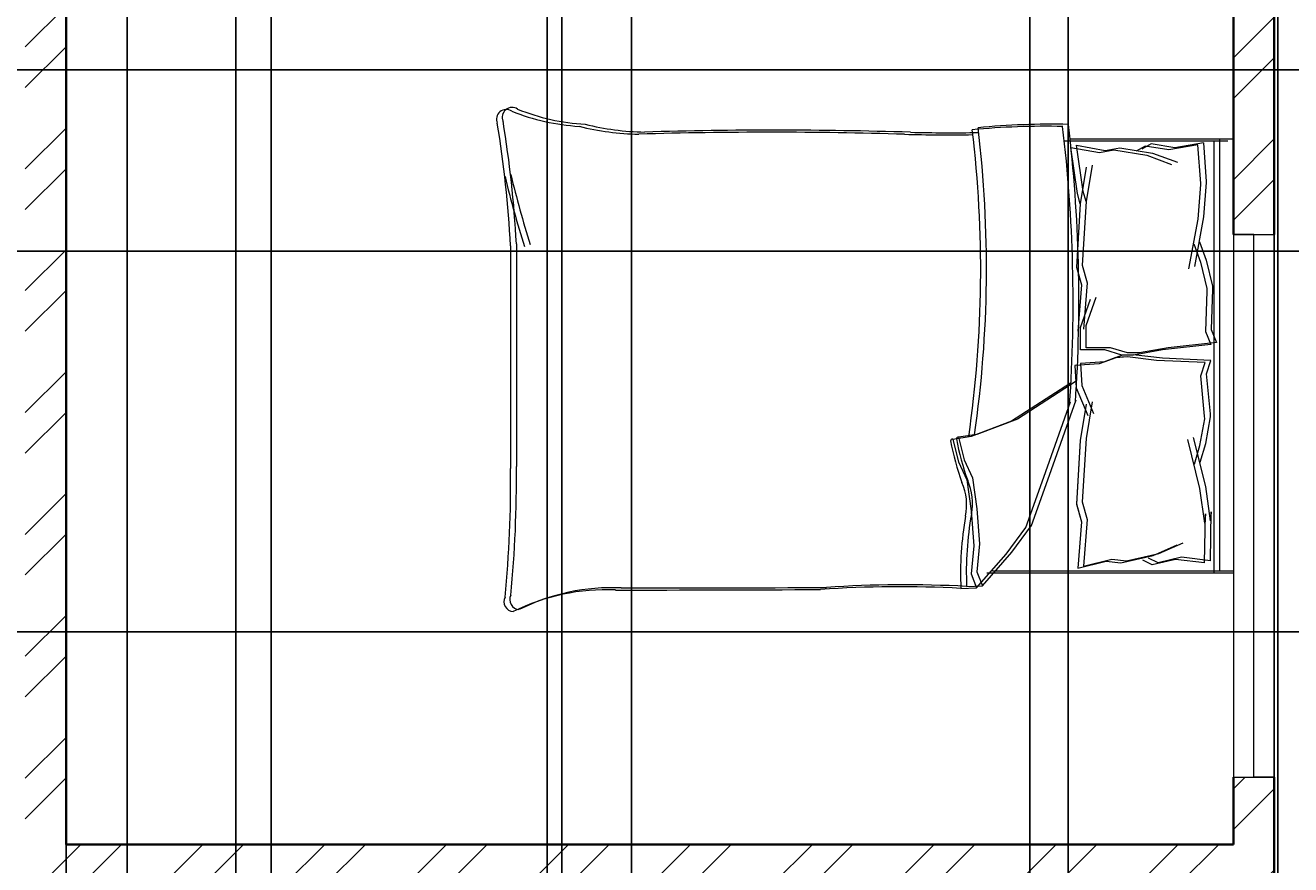
# Model space of a CAD drawing. Units: inches. Extents: x 2529 to 3014, y 1203 to 2262.
# Tile 8 of 13: x 2733 to 2873, y 1915 to 2008. Entities that reach past the tile are written whole.
import ezdxf

# ---------------------------------------------------------------- set-up
doc = ezdxf.new("R2010")
doc.units = ezdxf.units.IN
for name, color, linetype, lineweight in [('A-ANNO-DIMS', 2, 'Continuous', 18), ('A-FURN', 8, 'Continuous', 18), ('A-GLAZ', 191, 'Continuous', 18), ('A-WALL', 7, 'Continuous', 35), ('A-WALL-PATT', 143, 'Continuous', 13)]:
    doc.layers.add(name, color=color, linetype=linetype, lineweight=lineweight)
doc.styles.get("Standard").update_dxf_attribs({"font": 'arial.ttf'})
doc.dimstyles.get("Standard").update_dxf_attribs({"dimtxt": 0.18, "dimasz": 0.18, "dimexe": 0.18, "dimexo": 0.0625, "dimgap": 0.09, "dimtad": 0, "dimtih": 1, "dimtoh": 1, "dimdec": 4, "dimzin": 0, "dimdsep": 46, "dimtxsty": 'Standard', "dimcen": 0.09, "dimadec": 0, "dimazin": 0, "dimtfac": 1, "dimtdec": 4, "dimtofl": 0, "dimtmove": 0, "dimatfit": 3, "dimfxl": 1, "dimtolj": 1, "dimtzin": 0, "dimarcsym": 0})

# ---------------------------------------------------------------- blocks, each defined once
blk = doc.blocks.new('BED-DOUBLE')
for p, q in [((3.48, 63.33), (3.48, 81.44)), ((3.48, 63.33), (3.48, 81.44)), ((3.48, 81.44), (51.49, 81.44)), ((51.27, 81.44), (51.27, 54.83)), ((51.27, 81.44), (51.27, 54.83)), ((51.49, 81.44), (51.49, 80.8)), ((3.48, 79.91), (51.27, 79.91)), ((3.48, 79.91), (51.27, 79.91)), ((3.7, 62.69), (3.7, 80.8)), ((3.7, 62.69), (3.7, 80.8)), ((51.49, 80.8), (51.49, 54.19)), ((51.49, 80.8), (51.49, 54.19)), ((3.7, 79.27), (51.49, 79.27)), ((3.7, 79.27), (51.49, 79.27)), ((3.9, 78.11), (8.18, 78.43)), ((3.9, 78.11), (8.18, 78.43)), ((8.18, 78.43), (8.29, 78.42)), ((8.18, 78.43), (8.29, 78.42)), ((8.29, 78.42), (12.11, 78.13)), ((8.29, 78.42), (12.11, 78.13)), ((14.86, 77.69), (16.88, 78.42)), ((14.86, 77.69), (16.88, 78.42)), ((16.88, 78.42), (19.77, 79.14)), ((16.88, 78.42), (19.77, 79.14)), ((17.11, 77.78), (20, 78.5)), ((17.11, 77.78), (20, 78.5)), ((19.77, 79.14), (20.09, 79.14)), ((19.77, 79.14), (20.09, 79.14)), ((20, 78.5), (20.32, 78.5)), ((20, 78.5), (20.32, 78.5)), ((20.09, 79.14), (24.54, 78.99)), ((20.09, 79.14), (24.54, 78.99)), ((20.32, 78.5), (24.77, 78.36)), ((20.32, 78.5), (24.77, 78.36)), ((24.54, 78.99), (25.98, 79.57)), ((24.54, 78.99), (25.98, 79.57)), ((24.77, 78.36), (26.21, 78.93)), ((24.77, 78.36), (26.21, 78.93)), ((25.98, 79.57), (26.56, 74.22)), ((25.98, 79.57), (26.56, 74.22)), ((26.21, 78.93), (26.79, 73.58)), ((26.21, 78.93), (26.79, 73.58)), ((27.98, 78.95), (27.73, 73.58)), ((27.98, 78.95), (27.73, 73.58)), ((28.21, 78.31), (27.96, 72.94)), ((28.21, 78.31), (27.96, 72.94)), ((29.46, 78.46), (27.98, 78.95)), ((29.46, 78.46), (27.98, 78.95)), ((29.68, 77.83), (28.21, 78.31)), ((29.68, 77.83), (28.21, 78.31)), ((33.88, 78.89), (29.46, 78.46)), ((33.88, 78.89), (29.46, 78.46)), ((34.21, 78.91), (33.88, 78.89)), ((34.21, 78.91), (33.88, 78.89)), ((37.14, 78.37), (34.21, 78.91)), ((37.14, 78.37), (34.21, 78.91)), ((41.91, 78.37), (36.5, 77.02)), ((41.91, 78.37), (36.5, 77.02)), ((39.2, 77.77), (37.14, 78.37)), ((39.2, 77.77), (37.14, 78.37)), ((45.71, 78.9), (41.91, 78.37)), ((45.71, 78.9), (41.91, 78.37)), ((50.11, 78.89), (44.71, 78.98)), ((44.71, 78.98), (45.71, 78.9)), ((50.11, 78.89), (44.71, 78.98)), ((44.71, 78.98), (45.71, 78.9)), ((50.34, 78.25), (44.94, 78.34)), ((44.94, 78.34), (45.94, 78.26)), ((50.34, 78.25), (44.94, 78.34)), ((44.94, 78.34), (45.94, 78.26)), ((50.11, 78.89), (49.73, 75.68)), ((50.11, 78.89), (49.73, 75.68)), ((3.9, 78.13), (4.47, 74.95)), ((3.9, 78.13), (4.47, 74.95)), ((4.12, 77.49), (4.7, 74.31)), ((4.12, 77.49), (4.7, 74.31)), ((4.13, 77.47), (8.41, 77.8)), ((4.13, 77.47), (8.41, 77.8)), ((8.41, 77.8), (8.51, 77.78)), ((8.41, 77.8), (8.51, 77.78)), ((8.51, 77.78), (12.34, 77.49)), ((8.51, 77.78), (12.34, 77.49)), ((12.11, 78.13), (17.6, 77.12)), ((12.11, 78.13), (17.6, 77.12)), ((12.34, 77.49), (17.83, 76.48)), ((12.34, 77.49), (17.83, 76.48)), ((15.08, 77.05), (17.11, 77.78)), ((15.08, 77.05), (17.11, 77.78)), ((34.11, 78.25), (29.68, 77.83)), ((34.11, 78.25), (29.68, 77.83)), ((34.43, 78.27), (34.11, 78.25)), ((34.43, 78.27), (34.11, 78.25)), ((37.36, 77.73), (34.43, 78.27)), ((37.36, 77.73), (34.43, 78.27)), ((42.14, 77.73), (36.72, 76.38)), ((42.14, 77.73), (36.72, 76.38)), ((39.43, 77.13), (37.36, 77.73)), ((39.43, 77.13), (37.36, 77.73)), ((45.94, 78.26), (42.14, 77.73)), ((45.94, 78.26), (42.14, 77.73)), ((50.34, 78.25), (49.96, 75.04)), ((50.34, 78.25), (49.96, 75.04)), ((49.31, 73.19), (48.13, 75.87)), ((49.31, 73.19), (48.13, 75.87)), ((49.73, 75.68), (50.33, 73.11)), ((49.73, 75.68), (50.33, 73.11)), ((4.47, 74.95), (4.04, 72.34)), ((4.47, 74.95), (4.04, 72.34)), ((4.7, 74.31), (4.27, 71.7)), ((4.7, 74.31), (4.27, 71.7)), ((5.05, 72.49), (6.06, 75.24)), ((5.05, 72.49), (6.06, 75.24)), ((5.28, 71.85), (6.29, 74.6)), ((5.28, 71.85), (6.29, 74.6)), ((26.56, 74.22), (27.14, 71.04)), ((26.56, 74.22), (27.14, 71.04)), ((49.54, 72.55), (48.36, 75.23)), ((49.54, 72.55), (48.36, 75.23)), ((49.96, 75.04), (50.56, 72.47)), ((49.96, 75.04), (50.56, 72.47)), ((26.79, 73.58), (27.37, 70.4)), ((26.79, 73.58), (27.37, 70.4)), ((27.73, 73.58), (27.36, 70.37)), ((27.73, 73.58), (27.36, 70.37)), ((27.96, 72.94), (27.58, 69.73)), ((27.96, 72.94), (27.58, 69.73)), ((50.11, 69.61), (49.31, 73.19)), ((50.11, 69.61), (49.31, 73.19)), ((50.33, 73.11), (49.81, 72.06)), ((50.33, 73.11), (49.82, 72.06)), ((4.04, 72.34), (4.62, 71.33)), ((4.04, 72.34), (4.62, 71.33)), ((4.27, 71.7), (4.85, 70.69)), ((4.27, 71.7), (4.85, 70.69)), ((4.47, 68.87), (5.05, 72.49)), ((4.47, 68.87), (5.05, 72.49)), ((4.7, 68.23), (5.28, 71.85)), ((4.7, 68.23), (5.28, 71.85)), ((50.34, 68.98), (49.54, 72.55)), ((50.34, 68.98), (49.54, 72.55)), ((50.56, 72.47), (50.04, 71.42)), ((50.56, 72.47), (50.04, 71.42)), ((27.14, 71.04), (27.14, 69.74)), ((27.14, 71.04), (27.14, 69.74)), ((27.36, 70.37), (27.44, 69.07)), ((27.36, 70.37), (27.44, 69.07)), ((27.37, 70.4), (27.37, 69.1)), ((27.37, 70.4), (27.37, 69.1)), ((4.76, 67.28), (4.47, 68.87)), ((4.76, 67.28), (4.47, 68.87)), ((27.14, 69.74), (26.56, 67.86)), ((27.14, 69.74), (26.56, 67.86)), ((27.37, 69.1), (26.79, 67.22)), ((27.37, 69.1), (26.79, 67.22)), ((27.44, 69.07), (28.13, 67.23)), ((27.44, 69.07), (28.13, 67.23)), ((27.58, 69.73), (27.67, 68.43)), ((27.58, 69.73), (27.66, 68.43)), ((49.92, 68.01), (50.11, 69.61)), ((49.92, 68.01), (50.11, 69.61)), ((50.15, 67.37), (50.34, 68.98)), ((50.15, 67.37), (50.34, 68.98)), ((4.18, 64.1), (4.76, 67.28)), ((4.18, 64.1), (4.76, 67.28)), ((4.99, 66.64), (4.7, 68.23)), ((4.99, 66.64), (4.7, 68.23)), ((26.56, 67.86), (26.56, 65.18)), ((26.56, 67.86), (26.56, 65.18)), ((26.79, 67.22), (26.79, 64.54)), ((26.79, 67.22), (26.79, 64.54)), ((27.66, 68.43), (28.36, 66.59)), ((27.67, 68.43), (28.36, 66.59)), ((28.13, 67.23), (28.3, 64.55)), ((28.13, 67.23), (28.3, 64.55)), ((50.7, 64.87), (49.92, 68.01)), ((50.7, 64.87), (49.92, 68.01)), ((50.93, 64.23), (50.15, 67.37)), ((50.93, 64.23), (50.15, 67.37)), ((4.41, 63.46), (4.99, 66.64)), ((4.41, 63.46), (4.99, 66.64)), ((6.38, 65.81), (10.41, 65.15)), ((6.38, 65.81), (10.41, 65.15)), ((24.1, 65.18), (20.96, 66.27)), ((24.1, 65.18), (20.96, 66.27)), ((28.36, 66.59), (28.53, 63.91)), ((28.36, 66.59), (28.53, 63.91)), ((30.75, 64.7), (33.82, 65.99)), ((30.75, 64.7), (33.82, 65.99)), ((32.56, 65.81), (36.6, 65.15)), ((32.56, 65.81), (36.6, 65.15)), ((9.28, 64.83), (4.18, 64.1)), ((9.28, 64.83), (4.18, 64.1)), ((6.61, 65.18), (10.64, 64.51)), ((6.61, 65.18), (10.64, 64.51)), ((10.41, 65.15), (9.28, 64.83)), ((10.41, 65.15), (9.28, 64.83)), ((10.64, 64.51), (9.51, 64.19)), ((10.64, 64.51), (9.51, 64.19)), ((10.41, 65.15), (17.42, 64.72)), ((10.41, 65.15), (17.42, 64.72)), ((10.64, 64.51), (17.65, 64.08)), ((10.64, 64.51), (17.65, 64.08)), ((17.42, 64.72), (19.38, 65.27)), ((17.42, 64.72), (19.38, 65.27)), ((17.65, 64.08), (19.61, 64.64)), ((17.65, 64.08), (19.61, 64.64)), ((19.38, 65.27), (24.52, 64.87)), ((19.38, 65.27), (24.52, 64.87)), ((19.61, 64.64), (24.74, 64.23)), ((19.61, 64.64), (24.74, 64.23)), ((24.33, 64.54), (21.19, 65.63)), ((24.33, 64.54), (21.19, 65.63)), ((26.56, 65.18), (24.1, 65.18)), ((26.56, 65.18), (24.1, 65.18)), ((26.79, 64.54), (24.33, 64.54)), ((26.79, 64.54), (24.33, 64.54)), ((28.3, 64.55), (30.75, 64.7)), ((28.3, 64.55), (30.75, 64.7)), ((30.98, 64.06), (34.05, 65.35)), ((30.98, 64.06), (34.05, 65.35)), ((32.79, 65.18), (36.83, 64.51)), ((32.79, 65.18), (36.82, 64.51)), ((36.6, 65.15), (43.61, 64.72)), ((36.6, 65.15), (43.61, 64.72)), ((36.82, 64.51), (43.83, 64.08)), ((36.83, 64.51), (43.84, 64.08)), ((43.61, 64.72), (45.57, 65.27)), ((43.61, 64.72), (45.57, 65.27)), ((43.83, 64.08), (45.8, 64.64)), ((43.84, 64.08), (45.8, 64.64)), ((45.57, 65.27), (50.7, 64.87)), ((45.57, 65.27), (50.7, 64.87)), ((45.8, 64.64), (50.93, 64.23)), ((45.8, 64.64), (50.93, 64.23)), ((9.51, 64.19), (4.41, 63.46)), ((9.51, 64.19), (4.41, 63.46)), ((28.53, 63.91), (30.98, 64.06)), ((28.53, 63.91), (30.98, 64.06)), ((30.26, 64.06), (34.45, 57.57)), ((30.26, 64.06), (34.45, 57.57)), ((30.49, 63.42), (34.68, 56.93)), ((30.49, 63.42), (34.68, 56.93)), ((40.64, 61.13), (32.31, 64.06)), ((40.64, 61.13), (32.31, 64.06)), ((40.87, 60.49), (32.53, 63.42)), ((40.87, 60.49), (32.54, 63.42)), ((46.22, 59.11), (40.64, 61.13)), ((46.22, 59.11), (40.64, 61.13)), ((46.45, 58.48), (40.87, 60.49)), ((46.45, 58.48), (40.87, 60.49)), ((49.16, 56.95), (46.22, 59.11)), ((49.16, 56.95), (46.22, 59.11)), ((34.45, 57.57), (36.15, 53.08)), ((34.45, 57.57), (36.15, 53.08)), ((49.39, 56.31), (46.45, 58.48)), ((49.39, 56.31), (46.45, 58.48)), ((34.68, 56.93), (36.38, 52.44)), ((34.68, 56.93), (36.38, 52.44)), ((52.87, 53.7), (49.16, 56.95)), ((52.87, 53.7), (49.16, 56.95)), ((53.1, 53.06), (49.39, 56.31)), ((53.1, 53.06), (49.39, 56.31)), ((44.36, 53.08), (48.23, 53.39)), ((44.36, 53.08), (48.23, 53.39)), ((48.23, 53.39), (51.33, 53.08)), ((48.23, 53.39), (51.33, 53.08)), ((51.33, 53.08), (52.87, 53.7)), ((51.33, 53.08), (52.87, 53.7)), ((52.95, 51.95), (52.87, 53.7, 3.87)), ((52.95, 51.95), (52.87, 53.7, 3.87)), ((36.15, 53.08), (36.46, 51.07)), ((36.15, 53.08), (36.46, 51.07)), ((36.38, 52.44), (36.69, 50.43)), ((36.38, 52.44), (36.69, 50.43)), ((38.94, 51.69), (40.95, 52.61)), ((38.94, 51.69), (40.95, 52.61)), ((39.17, 51.05), (41.18, 51.97)), ((39.17, 51.05), (41.18, 51.97)), ((40.95, 52.61), (44.36, 53.08)), ((40.95, 52.61), (44.36, 53.08)), ((41.18, 51.97), (44.59, 52.44)), ((41.18, 51.97), (44.59, 52.44)), ((44.59, 52.44), (48.46, 52.75)), ((44.59, 52.44), (48.46, 52.75)), ((48.46, 52.75), (51.56, 52.44)), ((48.46, 52.75), (51.56, 52.44)), ((51.56, 52.44), (53.1, 53.06)), ((51.56, 52.44), (53.1, 53.06)), ((53.18, 51.31), (53.1, 53.06, 3.87)), ((53.18, 51.31), (53.1, 53.06, 3.87)), ((36.46, 51.07), (38.94, 51.69)), ((36.46, 51.07), (38.94, 51.69)), ((36.69, 50.43), (39.17, 51.05)), ((36.69, 50.43), (39.17, 51.05)), ((15.06, 2.2), (39.68, 2.2)), ((15.06, 2.2), (39.68, 2.2)), ((15.29, 1.56), (39.91, 1.56)), ((15.29, 1.56), (39.91, 1.56))]:
    blk.add_line(p, q)
for centre, radius, start, end in [((21.36, -100.61), 164.97, 86.0865, 96.7821), ((21.36, -100.61), 164.97, 86.0865, 96.7821), ((85.16, 61.35), 83.31, 178.7218, 185.604), ((85.16, 61.35), 83.31, 178.7218, 185.604), ((21.59, -101.25), 164.97, 86.0865, 96.7821), ((21.59, -101.25), 164.97, 86.0865, 96.7821), ((85.39, 60.71), 83.31, 178.7218, 185.604), ((85.39, 60.71), 83.31, 178.7218, 185.604), ((17.76, -74.87), 129.02, 81.7845, 96.9006), ((17.76, -74.87), 129.02, 81.7845, 96.9006), ((17.98, -75.51), 129.02, 81.7845, 96.9006), ((17.98, -75.51), 129.02, 81.7845, 96.9006), ((-167.31, 50.27), 170.11, 358.4762, 1.0082), ((-167.31, 50.27), 170.11, 358.4762, 1.0082), ((-167.08, 49.63), 170.11, 358.4762, 1.0082), ((-167.08, 49.63), 170.11, 358.4762, 1.0082), ((31.15, 79.96), 29.65, 280.6617, 289.8806), ((31.15, 79.96), 29.65, 280.6617, 289.8806), ((43.74, 46.38), 6.22, 78.6608, 113.7384), ((43.74, 46.38), 6.22, 78.6608, 113.7384), ((43.97, 45.74), 6.22, 78.6608, 113.7384), ((43.97, 45.74), 6.22, 78.6608, 113.7384), ((51.33, 88.1), 36.18, 259.8763, 272.5657), ((51.33, 88.1), 36.18, 259.8763, 272.5657), ((51.56, 87.46), 36.18, 259.8763, 272.5657), ((51.56, 87.46), 36.18, 259.8763, 272.5657), ((182.27, 45.13), 129.5, 176.9791, 183.8365), ((182.27, 45.13), 129.5, 176.9791, 183.8365), ((36.64, 51), 0.185, 160.2464, 271.1377), ((36.64, 51), 0.185, 160.2464, 271.1377), ((36.87, 50.36), 0.185, 160.2464, 271.1377), ((36.86, 50.36), 0.185, 160.2464, 271.1377), ((31.38, 79.32), 29.65, 280.6617, 289.8806), ((31.38, 79.32), 29.65, 280.6617, 289.8806), ((182.49, 44.49), 129.5, 176.9791, 183.8365), ((182.49, 44.49), 129.5, 176.9791, 183.8365), ((484.82, 30.83), 482.31, 178.2277, 181.7185), ((484.82, 30.83), 482.31, 178.2277, 181.7185), ((485.05, 30.19), 482.31, 178.2277, 181.7185), ((485.05, 30.19), 482.31, 178.2277, 181.7185), ((-4508.74, 13.62), 4561.86, 0.00217, 0.28689), ((-4508.74, 13.62), 4561.86, 0.00217, 0.28689), ((-4508.51, 12.98), 4561.86, 0.00217, 0.28689), ((-4508.51, 12.98), 4561.86, 0.00217, 0.28689), ((-26.9, 16.93), 29.63, 346.0648, 358.9113), ((-26.9, 16.93), 29.63, 346.0648, 358.9113), ((-26.67, 16.29), 29.63, 346.0648, 358.9113), ((-26.67, 16.29), 29.63, 346.0648, 358.9113), ((76.16, 12.78), 23.07, 177.4714, 206.4681), ((76.16, 12.78), 23.07, 177.4714, 206.4681), ((76.39, 12.14), 23.07, 177.4714, 206.4681), ((76.39, 12.14), 23.07, 177.4714, 206.4681), ((-21.66, 11.17), 23.56, 337.9751, 356.652), ((-21.66, 11.17), 23.56, 337.9751, 356.652), ((-21.43, 10.53), 23.56, 337.9751, 356.652), ((-21.43, 10.53), 23.56, 337.9751, 356.652), ((-17.22, 105.16), 106.46, 283.3832, 287.7053), ((-17.22, 105.16), 106.46, 283.3832, 287.7053), ((-16.99, 104.52), 106.46, 283.3832, 287.7053), ((-16.99, 104.52), 106.46, 283.3832, 287.7053), ((1.09, 1.73), 1.09, 146.1736, 293.4781), ((1.09, 1.73), 1.09, 146.1736, 293.4781), ((1.32, 1.09), 1.09, 146.1736, 293.4781), ((1.32, 1.09), 1.09, 146.1736, 293.4781), ((21.43, -119.39), 121.76, 92.9958, 99.4091), ((21.43, -119.39), 121.76, 92.9958, 99.4091), ((21.66, -120.03), 121.76, 92.9958, 99.4091), ((21.66, -120.03), 121.76, 92.9958, 99.4091), ((41.15, -130.83), 133.04, 84.4998, 90.6351), ((41.15, -130.83), 133.04, 84.4998, 90.6351), ((41.38, -131.47), 133.04, 84.4998, 90.6351), ((41.38, -131.47), 133.04, 84.4998, 90.6351), ((54.41, 2.57), 1.1, 242.6588, 356.02), ((54.41, 2.57), 1.1, 242.6588, 356.02), ((54.64, 1.93), 1.1, 242.6588, 356.02), ((54.64, 1.93), 1.1, 242.6588, 356.02)]:
    blk.add_arc(centre, radius, start, end)
blk = doc.blocks.new('*D36')
at = {"layer": 'A-ANNO-DIMS', "color": 0, "lineweight": -2, "transparency": 16777216}
for p, q in [((2737.56, 1582.57), (2737.56, 2243.11)), ((2737.74, 2242.93), (2746.49, 2242.93)), ((2756.15, 2242.93), (2747.4, 2242.93)), ((2756.33, 1582.57), (2756.33, 2243.11))]:
    blk.add_line(p, q, dxfattribs=at)
at = {"layer": 'A-ANNO-DIMS', "color": 0, "transparency": 16777216}
for points in [[(2737.74, 2242.96), (2737.74, 2242.9), (2737.56, 2242.93)], [(2756.15, 2242.96), (2756.15, 2242.9), (2756.33, 2242.93)]]:
    blk.add_solid(points, dxfattribs=at)
at = {"layer": 'Defpoints', "color": 0, "transparency": 16777216}
for p in [(2756.33, 2242.93), (2737.56, 1582.5), (2756.33, 1582.5)]:
    blk.add_point(p, dxfattribs=at)
at = {"layer": 'A-ANNO-DIMS', "color": 0, "transparency": 16777216, "insert": (2746.94, 2242.93), "char_height": 0.18, "attachment_point": 5}
blk.add_mtext('\\A1;18.778', dxfattribs=at)
blk = doc.blocks.new('*D37')
at = {"layer": 'A-ANNO-DIMS', "color": 0, "lineweight": -2, "transparency": 16777216}
for p, q in [((2756.33, 1582.57), (2756.33, 2243.11)), ((2756.51, 2242.93), (2774.11, 2242.93)), ((2792.15, 2242.93), (2774.55, 2242.93)), ((2792.33, 1582.57), (2792.33, 2243.11))]:
    blk.add_line(p, q, dxfattribs=at)
at = {"layer": 'A-ANNO-DIMS', "color": 0, "transparency": 16777216}
for points in [[(2756.51, 2242.96), (2756.51, 2242.9), (2756.33, 2242.93)], [(2792.15, 2242.96), (2792.15, 2242.9), (2792.33, 2242.93)]]:
    blk.add_solid(points, dxfattribs=at)
at = {"layer": 'Defpoints', "color": 0, "transparency": 16777216}
for p in [(2792.33, 2242.93), (2756.33, 1582.5), (2792.33, 1582.5)]:
    blk.add_point(p, dxfattribs=at)
at = {"layer": 'A-ANNO-DIMS', "color": 0, "transparency": 16777216, "insert": (2774.33, 2242.93), "char_height": 0.18, "attachment_point": 5}
blk.add_mtext('\\A1;36', dxfattribs=at)
blk = doc.blocks.new('*D38')
at = {"layer": 'A-ANNO-DIMS', "color": 0, "lineweight": -2, "transparency": 16777216}
for p, q in [((2844.06, 1582.57), (2844.06, 2243.11)), ((2844.24, 2242.93), (2857.35, 2242.93)), ((2871.26, 2242.93), (2858.14, 2242.93)), ((2871.44, 1582.57), (2871.44, 2243.11))]:
    blk.add_line(p, q, dxfattribs=at)
at = {"layer": 'A-ANNO-DIMS', "color": 0, "transparency": 16777216}
for points in [[(2844.24, 2242.96), (2844.24, 2242.9), (2844.06, 2242.93)], [(2871.26, 2242.96), (2871.26, 2242.9), (2871.44, 2242.93)]]:
    blk.add_solid(points, dxfattribs=at)
at = {"layer": 'Defpoints', "color": 0, "transparency": 16777216}
for p in [(2871.44, 2242.93), (2844.06, 1582.5), (2871.44, 1582.5)]:
    blk.add_point(p, dxfattribs=at)
at = {"layer": 'A-ANNO-DIMS', "color": 0, "transparency": 16777216, "insert": (2857.75, 2242.93), "char_height": 0.18, "attachment_point": 5}
blk.add_mtext('\\A1;27.39', dxfattribs=at)
blk = doc.blocks.new('*D39')
at = {"layer": 'A-ANNO-DIMS', "color": 0, "lineweight": -2, "transparency": 16777216}
for p, q in [((2848.27, 1734.07), (2848.27, 2243.11)), ((2848.45, 2242.93), (2864.3, 2242.93)), ((2881.08, 2242.93), (2865.23, 2242.93)), ((2881.26, 1734.07), (2881.26, 2243.11))]:
    blk.add_line(p, q, dxfattribs=at)
at = {"layer": 'A-ANNO-DIMS', "color": 0, "transparency": 16777216}
for points in [[(2848.45, 2242.96), (2848.45, 2242.9), (2848.27, 2242.93)], [(2881.08, 2242.96), (2881.08, 2242.9), (2881.26, 2242.93)]]:
    blk.add_solid(points, dxfattribs=at)
at = {"layer": 'Defpoints', "color": 0, "transparency": 16777216}
for p in [(2881.26, 2242.93), (2848.27, 1734), (2881.26, 1734)]:
    blk.add_point(p, dxfattribs=at)
at = {"layer": 'A-ANNO-DIMS', "color": 0, "transparency": 16777216, "insert": (2864.76, 2242.93), "char_height": 0.18, "attachment_point": 5}
blk.add_mtext('\\A1;32.994', dxfattribs=at)
blk = doc.blocks.new('*D40')
at = {"layer": 'A-ANNO-DIMS', "color": 0, "lineweight": -2, "transparency": 16777216}
for p, q in [((2744.32, 1738.57), (2744.32, 2243.11)), ((2744.5, 2242.93), (2771.84, 2242.93)), ((2799.84, 2242.93), (2772.49, 2242.93)), ((2800.02, 1738.57), (2800.02, 2243.11))]:
    blk.add_line(p, q, dxfattribs=at)
at = {"layer": 'A-ANNO-DIMS', "color": 0, "transparency": 16777216}
for points in [[(2744.5, 2242.96), (2744.5, 2242.9), (2744.32, 2242.93)], [(2799.84, 2242.96), (2799.84, 2242.9), (2800.02, 2242.93)]]:
    blk.add_solid(points, dxfattribs=at)
at = {"layer": 'Defpoints', "color": 0, "transparency": 16777216}
for p in [(2800.02, 2242.93), (2744.32, 1738.5), (2800.02, 1738.5)]:
    blk.add_point(p, dxfattribs=at)
at = {"layer": 'A-ANNO-DIMS', "color": 0, "transparency": 16777216, "insert": (2772.17, 2242.93), "char_height": 0.18, "attachment_point": 5}
blk.add_mtext('\\A1;55.7', dxfattribs=at)
blk = doc.blocks.new('*D57')
at = {"layer": 'A-ANNO-DIMS', "color": 0, "lineweight": -2, "transparency": 16777216}
for p, q in [((2871.06, 2198.44), (2871.06, 1483.77)), ((2893.92, 2198.44), (2893.92, 1483.77)), ((2871.24, 1483.95), (2882.02, 1483.95)), ((2893.74, 1483.95), (2882.95, 1483.95))]:
    blk.add_line(p, q, dxfattribs=at)
at = {"layer": 'A-ANNO-DIMS', "color": 0, "transparency": 16777216}
for points in [[(2871.24, 1483.98), (2871.24, 1483.92), (2871.06, 1483.95)], [(2893.74, 1483.98), (2893.74, 1483.92), (2893.92, 1483.95)]]:
    blk.add_solid(points, dxfattribs=at)
at = {"layer": 'Defpoints', "color": 0, "transparency": 16777216}
for p in [(2871.06, 2198.5), (2893.92, 2198.5), (2893.92, 1483.95)]:
    blk.add_point(p, dxfattribs=at)
at = {"layer": 'A-ANNO-DIMS', "color": 0, "transparency": 16777216, "insert": (2882.49, 1483.95), "char_height": 0.18, "attachment_point": 5}
blk.add_mtext('\\A1;22.866', dxfattribs=at)
blk = doc.blocks.new('*D60')
at = {"layer": 'A-ANNO-DIMS', "color": 0, "lineweight": -2, "transparency": 16777216}
for p, q in [((2918.49, 2003.13), (2541.45, 2003.13)), ((2541.63, 2002.95), (2541.63, 1993.28)), ((2541.63, 1983.24), (2541.63, 1992.91)), ((2918.49, 1983.06), (2541.45, 1983.06))]:
    blk.add_line(p, q, dxfattribs=at)
at = {"layer": 'A-ANNO-DIMS', "color": 0, "transparency": 16777216}
for points in [[(2541.6, 2002.95), (2541.66, 2002.95), (2541.63, 2003.13)], [(2541.6, 1983.24), (2541.66, 1983.24), (2541.63, 1983.06)]]:
    blk.add_solid(points, dxfattribs=at)
at = {"layer": 'Defpoints', "color": 0, "transparency": 16777216}
for p in [(2918.56, 2003.13), (2541.63, 1983.06), (2918.56, 1983.06)]:
    blk.add_point(p, dxfattribs=at)
at = {"layer": 'A-ANNO-DIMS', "color": 0, "transparency": 16777216, "insert": (2541.63, 1993.1), "char_height": 0.18, "attachment_point": 5}
blk.add_mtext('\\A1;20.077', dxfattribs=at)
blk = doc.blocks.new('*D61')
at = {"layer": 'A-ANNO-DIMS', "color": 0, "lineweight": -2, "transparency": 16777216}
for p, q in [((2918.49, 1983.06), (2541.45, 1983.06)), ((2541.63, 1982.88), (2541.63, 1962.21)), ((2541.63, 1941.18), (2541.63, 1961.85)), ((2918.49, 1941), (2541.45, 1941))]:
    blk.add_line(p, q, dxfattribs=at)
at = {"layer": 'A-ANNO-DIMS', "color": 0, "transparency": 16777216}
for points in [[(2541.6, 1982.88), (2541.66, 1982.88), (2541.63, 1983.06)], [(2541.6, 1941.18), (2541.66, 1941.18), (2541.63, 1941)]]:
    blk.add_solid(points, dxfattribs=at)
at = {"layer": 'Defpoints', "color": 0, "transparency": 16777216}
for p in [(2918.56, 1983.06), (2541.63, 1941), (2918.56, 1941)]:
    blk.add_point(p, dxfattribs=at)
at = {"layer": 'A-ANNO-DIMS', "color": 0, "transparency": 16777216, "insert": (2541.63, 1962.03), "char_height": 0.18, "attachment_point": 5}
blk.add_mtext('\\A1;42.05', dxfattribs=at)
blk = doc.blocks.new('*D78')
at = {"layer": 'A-ANNO-DIMS', "color": 0, "lineweight": -2, "transparency": 16777216}
for p, q in [((2760.22, 1599.16), (2760.22, 2243.11)), ((2760.4, 2242.93), (2775.15, 2242.93)), ((2790.54, 2242.93), (2775.8, 2242.93)), ((2790.72, 1599.16), (2790.72, 2243.11))]:
    blk.add_line(p, q, dxfattribs=at)
at = {"layer": 'A-ANNO-DIMS', "color": 0, "transparency": 16777216}
for points in [[(2760.4, 2242.96), (2760.4, 2242.9), (2760.22, 2242.93)], [(2790.54, 2242.96), (2790.54, 2242.9), (2790.72, 2242.93)]]:
    blk.add_solid(points, dxfattribs=at)
at = {"layer": 'Defpoints', "color": 0, "transparency": 16777216}
for p in [(2790.72, 2242.93), (2760.22, 1599.1), (2790.72, 1599.1)]:
    blk.add_point(p, dxfattribs=at)
at = {"layer": 'A-ANNO-DIMS', "color": 0, "transparency": 16777216, "insert": (2775.47, 2242.93), "char_height": 0.18, "attachment_point": 5}
blk.add_mtext('\\A1;30.5', dxfattribs=at)

msp = doc.modelspace()

# ---------------------------------------------------------------- hatches: boundary and pattern name
at = {"layer": 'A-WALL-PATT'}
h = msp.add_hatch(dxfattribs=at)
h.set_pattern_fill('ANSI32', color=256)
h.paths.add_polyline_path([(2686.5554, 2106.5032), (2622.0554, 2106.5032), (2622.0554, 2109.2964), (2617.4223, 2109.2964), (2613.0554, 2109.2964), (2613.0554, 2106.5032), (2577.0554, 2106.5032), (2577.0554, 2092.6918), (2586.0554, 2092.6918), (2586.0554, 2102.0032), (2682.0554, 2102.0032), (2682.0554, 2099.9833), (2686.5554, 2099.9833), (2686.5554, 2102.0032)])
h.paths.add_polyline_path([(2695.2249, 2054.0032), (2686.5554, 2054.0032), (2686.5554, 2080.2316), (2684.3054, 2080.2316), (2682.0554, 2080.2316), (2682.0554, 2054.0032), (2586.0554, 2054.0032), (2586.0554, 2068.6918), (2577.0554, 2068.6918), (2577.0554, 2019.1229), (2586.0554, 2019.1229), (2586.0554, 2049.5032), (2695.2249, 2049.5032)])
h.paths.add_polyline_path([(2737.5554, 2049.5032), (2866.5554, 2049.5032), (2866.5554, 2045.0233), (2871.0554, 2045.0233), (2871.0554, 2049.5032), (2871.0554, 2172.5032), (2866.5554, 2172.5032), (2829.1265, 2172.5032), (2829.1265, 2168.0032), (2866.5554, 2168.0032), (2866.5554, 2054.0032), (2737.5554, 2054.0032), (2737.5554, 2056.4892), (2735.3054, 2056.4892), (2733.0554, 2056.4892), (2733.0554, 2049.5032), (2733.0554, 1917.5032), (2733.0554, 1913.0032), (2871.0554, 1913.0032), (2871.0554, 1924.9149), (2868.8054, 1924.9149), (2866.5554, 1924.9149), (2866.5554, 1917.5032), (2737.5554, 1917.5032)], flags=17)
h.paths.add_polyline_path([(2972.0554, 2207.5032), (2613.0554, 2207.5032), (2613.0554, 2205.5032), (2613.0554, 2188.9366), (2622.0554, 2188.9366), (2622.0554, 2198.5032), (2733.0554, 2198.5032), (2733.0554, 2084.8053), (2735.3054, 2084.8053), (2737.5554, 2084.8053), (2737.5554, 2168.0032), (2769.1265, 2168.0032), (2769.1265, 2170.2532), (2769.1265, 2172.5032), (2737.5554, 2172.5032), (2737.5554, 2198.5032), (2963.0554, 2198.5032), (2963.0554, 2093.5032), (2912.0586, 2093.5032), (2912.0586, 2089.0032), (2918.5554, 2089.0032), (2918.5554, 2031.8749), (2923.0554, 2031.8749), (2923.0554, 2089.0032), (2963.0554, 2089.0032), (2963.0554, 2010.0032), (2923.0554, 2010.0032), (2923.0554, 2011.9417), (2918.5554, 2011.9417), (2918.5554, 2003.1338), (2923.0554, 2003.1338), (2923.0554, 2005.5032), (2963.0554, 2005.5032), (2963.0554, 1917.5032), (2963.0554, 1691.0776), (2972.0554, 1691.0776), (2972.0554, 1917.5032)])
h.paths.add_polyline_path([(2963.0554, 1945.5032), (2923.0554, 1945.5032), (2923.0554, 1983.0571), (2920.8054, 1983.0571), (2918.5554, 1983.0571), (2918.5554, 1941.0032), (2963.0554, 1941.0032)], flags=17)
h.paths.add_polyline_path([(2930.3679, 1788.7532), (2930.3679, 1791.0032), (2894.8637, 1791.0032), (2894.8637, 1786.5032), (2900.5554, 1786.5032), (2900.5554, 1784.6931), (2905.0554, 1784.6931), (2905.0554, 1786.5032), (2930.3679, 1786.5032)], flags=17)
h.paths.add_polyline_path([(2963.0554, 1791.0032), (2954.3679, 1791.0032), (2954.3679, 1786.5032), (2963.0554, 1786.5032)], flags=17)
h.paths.add_polyline_path([(2871.0554, 1853.0032), (2919.0554, 1853.0032), (2919.0554, 1847.0972), (2923.5554, 1847.0972), (2923.5554, 1853.0032), (2923.5554, 1857.5032), (2871.0554, 1857.5032), (2871.0554, 1871.7024), (2866.5554, 1871.7024), (2866.5554, 1791.0032), (2737.5554, 1791.0032), (2737.5554, 1806.6712), (2735.3054, 1806.6712), (2733.0554, 1806.6712), (2733.0554, 1791.0032), (2733.0554, 1786.5032), (2733.0554, 1780.6235), (2737.5554, 1780.6235), (2737.5554, 1786.5032), (2872.8745, 1786.5032), (2872.8745, 1788.7532), (2872.8745, 1791.0032), (2871.0554, 1791.0032)], flags=17)
h.paths.add_polyline_path([(2844.0554, 1734.0032), (2848.2652, 1734.0032), (2848.2652, 1738.5032), (2800.0167, 1738.5032), (2800.0167, 1734.0032), (2839.5554, 1734.0032), (2839.5554, 1582.5032), (2792.3334, 1582.5032), (2792.3334, 1573.5032), (2871.4433, 1573.5032), (2871.4433, 1578.0032), (2871.4433, 1582.5032), (2844.0554, 1582.5032)])
h.paths.add_polyline_path([(2972.0554, 1631.0776), (2963.0554, 1631.0776), (2963.0554, 1582.5032), (2931.4433, 1582.5032), (2931.4433, 1573.5032), (2972.0554, 1573.5032)])
h.paths.add_polyline_path([(2756.3334, 1582.5032), (2737.5554, 1582.5032), (2737.5554, 1734.0032), (2744.3201, 1734.0032), (2744.3201, 1738.5032), (2737.5554, 1738.5032), (2737.5554, 1746.0094), (2733.0554, 1746.0094), (2733.0554, 1738.5032), (2733.0554, 1612.5032), (2728.2475, 1612.5032), (2728.2475, 1603.5032), (2733.0554, 1603.5032), (2733.0554, 1582.5032), (2733.0554, 1573.5032), (2756.3334, 1573.5032), (2756.3334, 1578.0032)])
h.paths.add_polyline_path([(2695.7662, 1612.5032), (2658.4771, 1612.5032), (2658.4771, 1603.5032), (2695.7662, 1603.5032), (2695.7662, 1608.0032)])
h.paths.add_polyline_path([(2586.0554, 1686.9483), (2577.0554, 1686.9483), (2577.0554, 1603.5032), (2598.4771, 1603.5032), (2598.4771, 1608.0032), (2598.4771, 1612.5032), (2586.0554, 1612.5032)])
h.paths.add_polyline_path([(2683.2727, 1791.0032), (2586.0554, 1791.0032), (2586.0554, 1815.6736), (2581.5554, 1815.6736), (2577.0554, 1815.6736), (2577.0554, 1746.9483), (2586.0554, 1746.9483), (2586.0554, 1786.5032), (2683.2727, 1786.5032)])
h.paths.add_polyline_path([(2586.0554, 1959.1229), (2577.0554, 1959.1229), (2577.0554, 1875.6736), (2586.0554, 1875.6736), (2586.0554, 1913.0032), (2683.2727, 1913.0032), (2683.2727, 1917.5032), (2586.0554, 1917.5032)])
h = msp.add_hatch(dxfattribs=at)
h.set_pattern_fill('ANSI32', color=256)
h.paths.add_polyline_path([(2871.0554, 2017.2091), (2868.8054, 2017.2091), (2866.5554, 2017.2091), (2866.5554, 1984.9149), (2871.0554, 1984.9149)])
h.paths.add_polyline_path([(2755.9438, 2027.3569), (2794.7842, 2027.3569), (2794.7842, 2046.0142), (2755.9438, 2046.0142)], flags=9)

# ---------------------------------------------------------------- linework, layer by layer
at = {"layer": 'A-GLAZ'}
for p, q in [((2868.8054, 1984.9149), (2866.5554, 1984.9149)), ((2866.5554, 1984.9149), (2871.0554, 1984.9149)), ((2866.5554, 1984.9149), (2866.5554, 1924.9149)), ((2868.8054, 1924.9149), (2868.8054, 1984.9149)), ((2871.0554, 1984.9149), (2871.0554, 1924.9149)), ((2866.5554, 1924.9149), (2871.0554, 1924.9149)), ((2871.0554, 1924.9149), (2868.8054, 1924.9149))]:
    msp.add_line(p, q, dxfattribs=at)
at = {"layer": 'A-WALL'}
for p, q in [((2737.5554, 2049.5032), (2737.5554, 1917.5032)), ((2866.5554, 2018.3735), (2866.5554, 1984.9149)), ((2871.0554, 2017.2091), (2871.0554, 1984.9149)), ((2866.5554, 1924.9149), (2866.5554, 1917.5032)), ((2871.0554, 1924.9149), (2871.0554, 1913.0032)), ((2737.5554, 1917.5032), (2866.5554, 1917.5032))]:
    msp.add_line(p, q, dxfattribs=at)

# ---------------------------------------------------------------- block references
at = {"layer": 'A-FURN', "rotation": 269.9999998331855}
msp.add_blockref('BED-DOUBLE', (2785.1118, 1998.9661), dxfattribs=at)

# ---------------------------------------------------------------- dimensions: what is measured, and where the dimension line sits
at = {"layer": 'A-ANNO-DIMS'}
for base, p1, p2, override, picture, middle in [((2756.3334, 2242.9282), (2737.5554, 1582.5032), (2756.3334, 1582.5032), {"dimdec": 3, "dimlfac": 1, "dimrnd": 0, "dimzin": 0, "dimdsep": 46, "dimlunit": 2}, '*D36', (2746.9444, 2242.9282)), ((2800.0167, 2242.9282), (2744.3201, 1738.5032), (2800.0167, 1738.5032), {"dimdec": 1, "dimlfac": 1, "dimrnd": 0, "dimzin": 0, "dimdsep": 46, "dimlunit": 2}, '*D40', (2772.1684, 2242.9282)), ((2792.3334, 2242.9282), (2756.3334, 1582.5032), (2792.3334, 1582.5032), {"dimdec": 0, "dimlfac": 1, "dimrnd": 0, "dimzin": 0, "dimdsep": 46, "dimlunit": 2}, '*D37', (2774.3334, 2242.9282)), ((2790.721, 2242.9282), (2760.2227, 1599.0994), (2790.721, 1599.0994), {"dimdec": 1, "dimlfac": 1, "dimrnd": 0, "dimzin": 0, "dimdsep": 46, "dimlunit": 2}, '*D78', (2775.4718, 2242.9282)), ((2871.4433, 2242.9282), (2844.0554, 1582.5032), (2871.4433, 1582.5032), {"dimdec": 2, "dimlfac": 1, "dimrnd": 0, "dimzin": 0, "dimdsep": 46, "dimlunit": 2}, '*D38', (2857.7493, 2242.9282)), ((2881.259, 2242.9282), (2848.2652, 1734.0032), (2881.259, 1734.0032), {"dimdec": 3, "dimlfac": 1, "dimrnd": 0, "dimzin": 0, "dimdsep": 46, "dimlunit": 2}, '*D39', (2864.7621, 2242.9282)), ((2893.9216, 1483.9492), (2871.0554, 2198.5032), (2893.9216, 2198.5032), {"dimdec": 3, "dimlfac": 1, "dimrnd": 0, "dimzin": 0, "dimdsep": 46, "dimlunit": 2}, '*D57', (2882.4885, 1483.9492))]:
    dim = msp.add_linear_dim(base=base, p1=p1, p2=p2, dimstyle='Standard', override=override, dxfattribs=at)
    dim.commit()
    dim.dimension.update_dxf_attribs({"geometry": picture, "text_midpoint": middle})
for base, p1, p2, override, picture, middle in [((2541.6304, 1983.0571), (2918.5554, 2003.1338), (2918.5554, 1983.0571), {"dimdec": 3, "dimlfac": 1, "dimrnd": 0, "dimzin": 0, "dimdsep": 46, "dimlunit": 2}, '*D60', (2541.6304, 1993.0955)), ((2541.6304, 1941.0032), (2918.5554, 1983.0571), (2918.5554, 1941.0032), {"dimdec": 2, "dimlfac": 1, "dimrnd": 0, "dimzin": 0, "dimdsep": 46, "dimlunit": 2}, '*D61', (2541.6304, 1962.0302))]:
    dim = msp.add_linear_dim(base=base, p1=p1, p2=p2, angle=90, dimstyle='Standard', override=override, dxfattribs=at)
    dim.commit()
    dim.dimension.update_dxf_attribs({"geometry": picture, "text_midpoint": middle})

doc.saveas('drawing.dxf')
